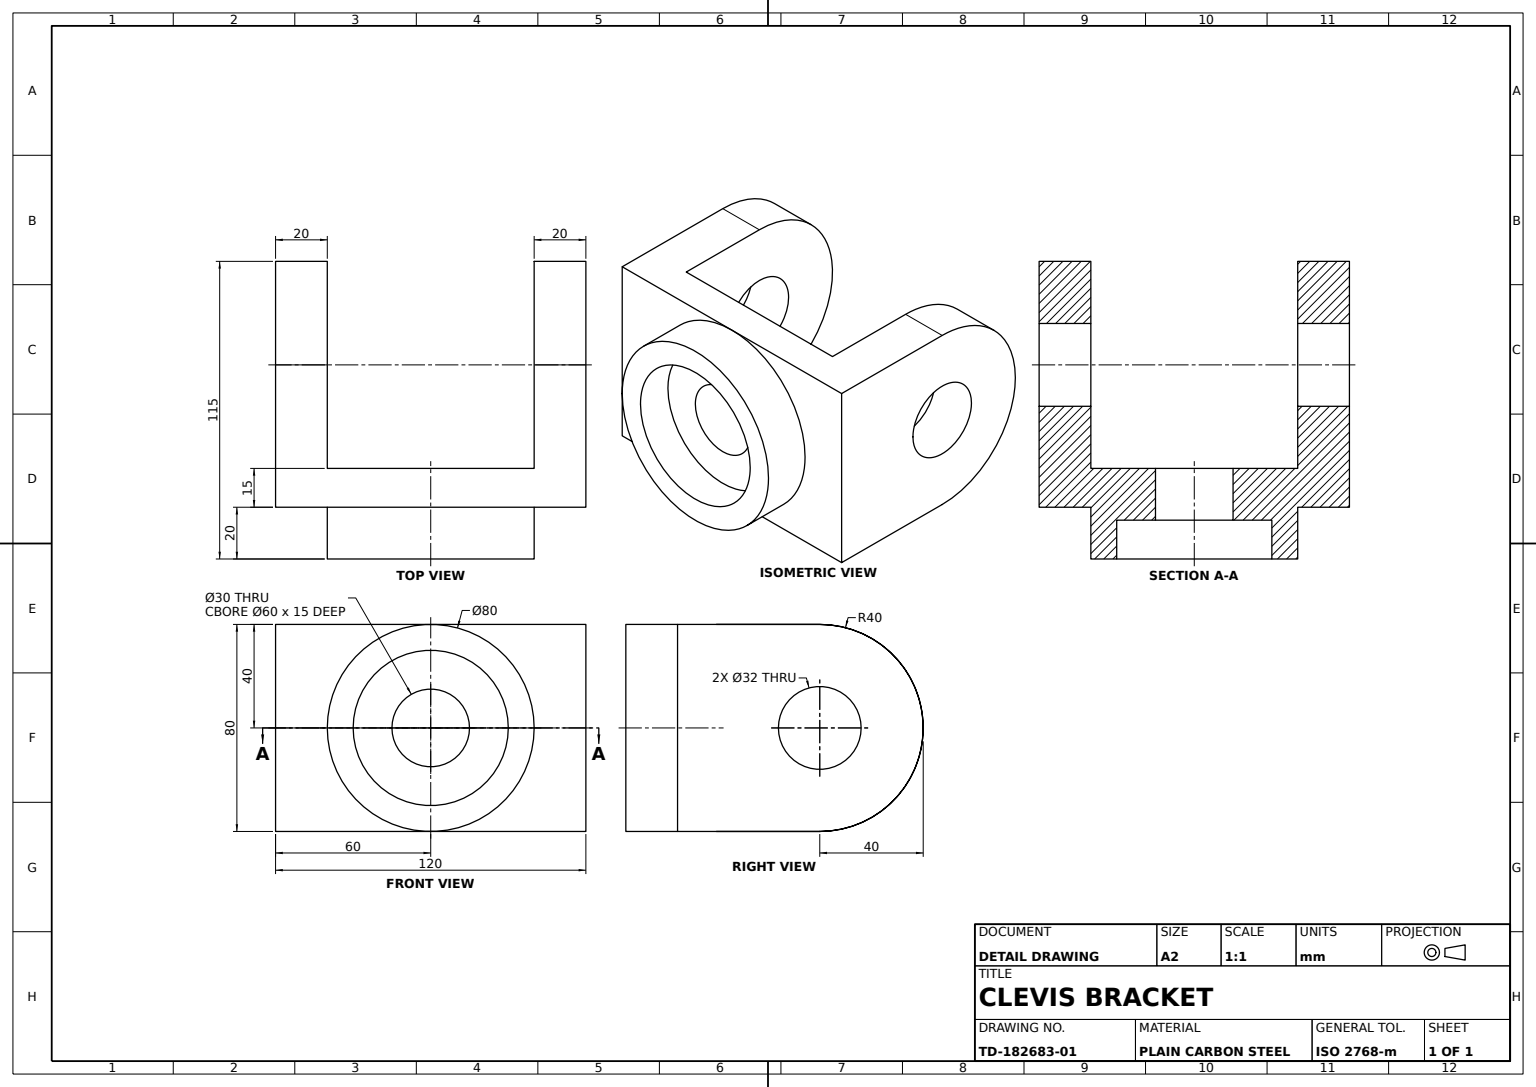
from build123d import *

# Parameters (mm, degrees)
BASE_PLATE_SKETCH_W        = 120
BASE_PLATE_SKETCH_H        = 80
BASE_PLATE_120X80X15_DEPTH = 15
BORE_30_SKETCH_R           = 15
BORE_30_DEPTH              = 15
HUB_BOSS_SKETCH_R          = 40
HUB_BOSS_SKETCH_R_2        = 30
HUB_BOSS_DEPTH             = 20
HUB_INNER_STEP_SKETCH_R    = 30
HUB_INNER_STEP_SKETCH_R_2  = 15
HUB_INNER_STEP_DEPTH       = 5
LUG_A_SKETCH_R             = 16
LUG_A_DEPTH                = 20
LUG_START                  = -20
LUG_B_SKETCH_R             = 16
LUG_B_DEPTH                = 20


with BuildPart() as part:
    # Base Plate Sketch → Base Plate 120x80x15 (new body)
    with BuildSketch(Plane.XY):
        Rectangle(BASE_PLATE_SKETCH_W, BASE_PLATE_SKETCH_H)
    extrude(amount=BASE_PLATE_120X80X15_DEPTH)

    # Bore Ø30 Sketch → Bore Ø30 (cut)
    with BuildSketch(Plane(origin=(0, 0, 0), x_dir=(-1, 0, 0), z_dir=(0, 0, -1))):
        Circle(BORE_30_SKETCH_R)
    extrude(amount=-BORE_30_DEPTH, mode=Mode.SUBTRACT)

    # Hub Boss Sketch → Hub Boss (add)
    with BuildSketch(Plane.XY.offset(15)):
        with Locations(Location((0, 0, 0), (0, 0, 270))):
            Circle(HUB_BOSS_SKETCH_R)
        Circle(HUB_BOSS_SKETCH_R_2, mode=Mode.SUBTRACT)
    extrude(amount=HUB_BOSS_DEPTH)

    # Hub Inner Step Sketch → Hub Inner Step (add)
    with BuildSketch(Plane.XY.offset(15)):
        Circle(HUB_INNER_STEP_SKETCH_R)
        with Locations(Location((0, 0, 0), (0, 0, 180))):
            Circle(HUB_INNER_STEP_SKETCH_R_2, mode=Mode.SUBTRACT)
    extrude(amount=HUB_INNER_STEP_DEPTH)

    # Lug A Sketch → Lug A (add)
    with BuildSketch(Plane(origin=(60, 0, 0), x_dir=(0, 0, -1), z_dir=(1, 0, 0))):
        with BuildLine():
            Line((0, 40), (40, 40))
            ThreePointArc((40, 40), (80, 0), (40, -40))
            Line((40, -40), (0, -40))
            Line((0, -40), (0, 40))
        make_face()
        with Locations((40, 0)):
            Circle(LUG_A_SKETCH_R, mode=Mode.SUBTRACT)
    extrude(amount=-LUG_A_DEPTH)

    # Lug B Sketch → Lug B (add)
    with BuildSketch(Plane.ZY.offset(60).offset(LUG_START)):
        with BuildLine():
            Line((-40, 40), (15, 40))
            Line((15, 40), (15, -40))
            Line((15, -40), (-40, -40))
            ThreePointArc((-40, -40), (-80, 0), (-40, 40))
        make_face()
        with Locations(Location((-40, 0, 0), (0, 0, 180))):
            Circle(LUG_B_SKETCH_R, mode=Mode.SUBTRACT)
    extrude(amount=LUG_B_DEPTH)


solid = part.part
